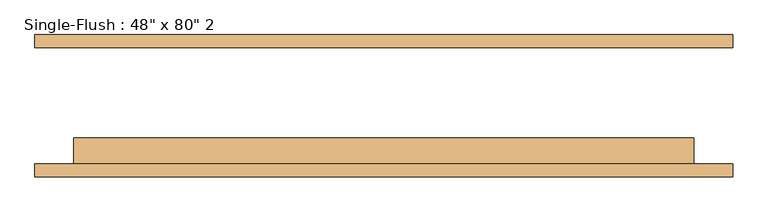
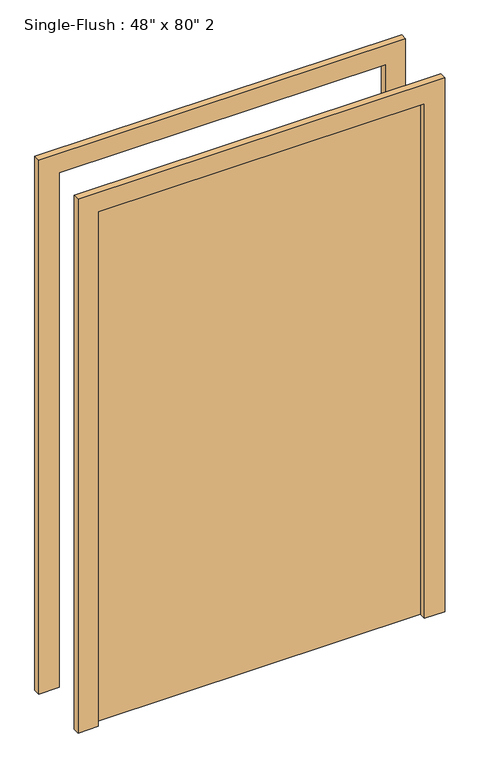
"""IFC4 building model written with IfcOpenShell, lengths in millimetres: door geometry."""

from ifc_helpers import new_model, si_unit, frame, origin, origin_with_axes, place, context, project, spatial, polyline, outline, extrude, source, transform, mapped, element, save


def door_6982a541(model_context):
    return source(origin(), model_context, "Body", "SweptSolid", [
        extrude(outline(polyline([(2108.2, -685.8), (0.0, -685.8), (0.0, -609.6), (2032.0, -609.6), (2032.0, 609.6), (0.0, 609.6), (0.0, 685.8), (2108.2, 685.8), (2108.2, -685.8)])), frame((0.0, -139.7, 0.0), z_axis=(0.0, 1.0, 0.0), x_axis=(0.0, 0.0, 1.0)), (0.0, 0.0, 1.0), 25.4),
        extrude(outline(polyline([(2108.2, 685.8), (2108.2, -685.8), (0.0, -685.8), (0.0, -609.6), (2032.0, -609.6), (2032.0, 609.6), (0.0, 609.6), (0.0, 685.8), (2108.2, 685.8)])), frame((0.0, 114.3, 0.0), z_axis=(0.0, 1.0, 0.0), x_axis=(0.0, 0.0, 1.0)), (0.0, 0.0, 1.0), 25.4),
        extrude(outline(polyline([(609.6, -63.5), (609.6, -114.3), (-609.6, -114.3), (-609.6, -63.5), (609.6, -63.5)])), origin_with_axes(), (0.0, 0.0, 1.0), 2032.0),
    ])


if __name__ == "__main__":
    model = new_model("IFC4")
    model_context = context("Model", 3, world=origin())
    ifc_project = project(units=[si_unit("LENGTHUNIT", "METRE", prefix="MILLI")], contexts=[model_context])
    site = spatial("IfcSite", under=ifc_project)
    building = spatial("IfcBuilding", under=site)
    placement = place(None, origin())
    door_shape = door_6982a541(model_context)
    element("IfcDoor", 1, ObjectType="Single-Flush : 48\" x 80\" 2", at=placement, inside=building, context=model_context, shape_type="MappedRepresentation", body=[
        mapped(door_shape, transform((0.0, 0.0, 0.0), x_axis=(1.0, 0.0, 0.0), y_axis=(0.0, 1.0, 0.0), z_axis=(0.0, 0.0, 1.0))),
    ])
    save(model, "model.ifc")

# Revit data of these elements
# Type "Single-Flush : 48\" x 80\" 2"
#   Type Mark = "16"
#   Construction Type Id = "MDOOR"
#   Assembly Code = "C1020"
#   Analytic Construction = "Metal"
#   Thickness = 0' - 2"
#   Heat Transfer Coefficient (U) = 0.651978 BTU/(h·ft²·°F)
#   Height = 6' - 8"
#   Trim Projection Ext = 0' - 1"
#   Trim Projection Int = 0' - 1"
#   Trim Width = 0' - 3"
#   Width = 4' - 0"
#   Define Thermal Properties by = 1
#   Door Material = Door - Panel
#   Frame Material = Door - Frame
#   Visual Light Transmittance = 0
#   Solar Heat Gain Coefficient = 0
#   Function = (empty or 0)
#   Wall Closure = (empty or 0)
# Element 1 (IfcDoor, "Single-Flush : 48\" x 80\" 2")
#   Materials on its faces: "Door - Frame", "Door - Panel"
# Materials
#   "Door - Panel": class "Wood", colour RGB 210 159 95, transparency 0, Cost = 0
#   "Door - Frame": colour RGB 118 70 51, transparency 0, Cost = 0
